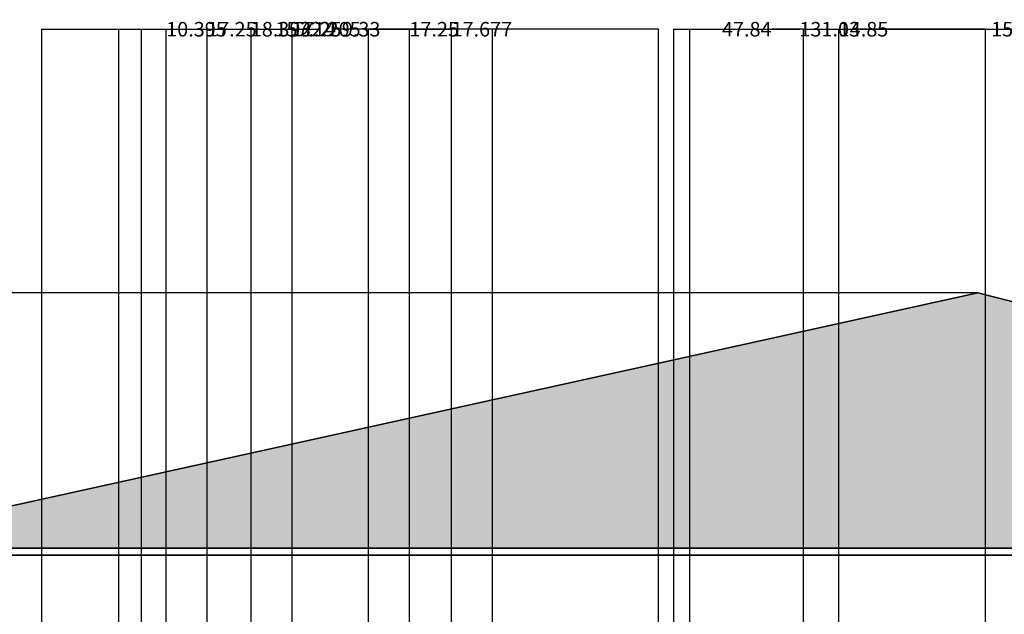
# Model space of a CAD drawing. Units: inches. Extents: x -655 to 499, y 20 to 616.
# Tile 5 of 7: x -409 to 5, y 365 to 616. Entities that reach past the tile are written whole.
import ezdxf

# ---------------------------------------------------------------- set-up
doc = ezdxf.new("R2010")
doc.units = ezdxf.units.IN
doc.header["$MEASUREMENT"] = 0
doc.layers.add('A-ANNO-DIMS', color=2, linetype='Continuous', lineweight=18)
doc.layers.add('A-ROOF', color=1, linetype='Continuous', lineweight=35)
doc.styles.get("Standard").update_dxf_attribs({"font": 'arial.ttf'})
doc.dimstyles.get("Standard").update_dxf_attribs({"dimtxt": 6.125, "dimasz": 0.18, "dimexe": 0.18, "dimexo": 0.0625, "dimgap": 0.09, "dimtad": 0, "dimtih": 1, "dimtoh": 1, "dimdec": 4, "dimzin": 0, "dimdsep": 46, "dimlunit": 4, "dimtxsty": 'Standard', "dimcen": 0.09, "dimadec": 0, "dimazin": 0, "dimtfac": 1, "dimtdec": 4, "dimtofl": 0, "dimtmove": 0, "dimatfit": 3, "dimfxl": 1, "dimtolj": 1, "dimtzin": 0, "dimarcsym": 0})

# ---------------------------------------------------------------- blocks, each defined once
blk = doc.blocks.new('*D10')
at = {"layer": 'A-ANNO-DIMS', "color": 0, "lineweight": -2, "transparency": 16777216}
for p, q in [((434.11, 393.11), (434.11, 23.7)), ((-590.16, 75.57), (-590.16, 23.7)), ((-589.98, 23.88), (-90.54, 23.88)), ((433.93, 23.88), (-65.51, 23.88))]:
    blk.add_line(p, q, dxfattribs=at)
at = {"layer": 'A-ANNO-DIMS', "color": 0, "transparency": 16777216}
for points in [[(-589.98, 23.91), (-589.98, 23.85), (-590.16, 23.88)], [(433.93, 23.91), (433.93, 23.85), (434.11, 23.88)]]:
    blk.add_solid(points, dxfattribs=at)
at = {"layer": 'Defpoints', "color": 0, "transparency": 16777216}
for p in [(434.11, 393.17), (-590.16, 75.63), (434.11, 23.88)]:
    blk.add_point(p, dxfattribs=at)
at = {"layer": 'A-ANNO-DIMS', "color": 0, "transparency": 16777216, "insert": (-78.02, 23.88), "char_height": 6.125, "attachment_point": 5}
blk.add_mtext('\\A1;1024.3', dxfattribs=at)
blk = doc.blocks.new('*D17')
at = {"layer": 'A-ANNO-DIMS', "color": 0, "lineweight": -2, "transparency": 16777216}
for p, q in [((-399.38, 249.9), (-399.38, 611.71)), ((-399.2, 611.53), (-282.57, 611.53)), ((-140.23, 611.53), (-256.86, 611.53)), ((-140.05, 249.9), (-140.05, 611.71))]:
    blk.add_line(p, q, dxfattribs=at)
at = {"layer": 'A-ANNO-DIMS', "color": 0, "transparency": 16777216}
for points in [[(-399.2, 611.56), (-399.2, 611.5), (-399.38, 611.53)], [(-140.23, 611.56), (-140.23, 611.5), (-140.05, 611.53)]]:
    blk.add_solid(points, dxfattribs=at)
at = {"layer": 'Defpoints', "color": 0, "transparency": 16777216}
for p in [(-140.05, 611.53), (-399.38, 249.84), (-140.05, 249.84)]:
    blk.add_point(p, dxfattribs=at)
at = {"layer": 'A-ANNO-DIMS', "color": 0, "transparency": 16777216, "insert": (-269.71, 611.53), "char_height": 6.125, "attachment_point": 5}
blk.add_mtext('\\A1;259.33', dxfattribs=at)
blk = doc.blocks.new('*D21')
at = {"layer": 'A-ANNO-DIMS', "color": 0, "lineweight": -2, "transparency": 16777216}
for p, q in [((179.11, 559.78), (486.04, 559.78)), ((485.86, 559.6), (485.86, 320.92)), ((485.86, 75.81), (485.86, 314.49)), ((-590.1, 75.63), (486.04, 75.63))]:
    blk.add_line(p, q, dxfattribs=at)
at = {"layer": 'A-ANNO-DIMS', "color": 0, "transparency": 16777216}
for points in [[(485.83, 559.6), (485.89, 559.6), (485.86, 559.78)], [(485.83, 75.81), (485.89, 75.81), (485.86, 75.63)]]:
    blk.add_solid(points, dxfattribs=at)
at = {"layer": 'Defpoints', "color": 0, "transparency": 16777216}
for p in [(179.05, 559.78), (485.86, 559.78), (-590.16, 75.63)]:
    blk.add_point(p, dxfattribs=at)
at = {"layer": 'A-ANNO-DIMS', "color": 0, "transparency": 16777216, "insert": (485.86, 317.7), "char_height": 6.125, "attachment_point": 5}
blk.add_mtext('\\A1;484.15', dxfattribs=at)
blk = doc.blocks.new('*D22')
at = {"layer": 'A-ANNO-DIMS', "color": 0, "lineweight": -2, "transparency": 16777216}
for p, q in [((-5.81, 500.52), (-642.09, 500.52)), ((-641.91, 500.34), (-641.91, 450.03)), ((-641.91, 393.29), (-641.91, 443.6)), ((-493.1, 393.11), (-642.09, 393.11))]:
    blk.add_line(p, q, dxfattribs=at)
at = {"layer": 'A-ANNO-DIMS', "color": 0, "transparency": 16777216}
for points in [[(-641.94, 500.34), (-641.88, 500.34), (-641.91, 500.52)], [(-641.94, 393.29), (-641.88, 393.29), (-641.91, 393.11)]]:
    blk.add_solid(points, dxfattribs=at)
at = {"layer": 'Defpoints', "color": 0, "transparency": 16777216}
for p in [(-641.91, 500.52), (-5.74, 500.52), (-493.03, 393.11)]:
    blk.add_point(p, dxfattribs=at)
at = {"layer": 'A-ANNO-DIMS', "color": 0, "transparency": 16777216, "insert": (-641.91, 446.81), "char_height": 6.125, "attachment_point": 5}
blk.add_mtext('\\A1;107.41', dxfattribs=at)
blk = doc.blocks.new('*D27')
at = {"layer": 'A-ANNO-DIMS', "color": 0, "lineweight": -2, "transparency": 16777216}
for p, q in [((-357.43, 359.35), (-357.43, 611.71)), ((-357.25, 611.53), (-347.21, 611.53)), ((-347.03, 350.2), (-347.03, 611.71)), ((-347.03, 611.53), (-346.85, 611.53))]:
    blk.add_line(p, q, dxfattribs=at)
at = {"layer": 'A-ANNO-DIMS', "color": 0, "transparency": 16777216}
for points in [[(-357.25, 611.56), (-357.25, 611.5), (-357.43, 611.53)], [(-347.21, 611.56), (-347.21, 611.5), (-347.03, 611.53)]]:
    blk.add_solid(points, dxfattribs=at)
at = {"layer": 'Defpoints', "color": 0, "transparency": 16777216}
for p in [(-347.03, 611.53), (-357.43, 359.29), (-347.03, 350.13)]:
    blk.add_point(p, dxfattribs=at)
at = {"layer": 'A-ANNO-DIMS', "color": 0, "transparency": 16777216, "insert": (-334.32, 611.53), "char_height": 6.125, "attachment_point": 5}
blk.add_mtext('\\A1;10.395', dxfattribs=at)
blk = doc.blocks.new('*D28')
at = {"layer": 'A-ANNO-DIMS', "color": 0, "lineweight": -2, "transparency": 16777216}
for p, q in [((-347.03, 350.2), (-347.03, 611.71)), ((-346.85, 611.53), (-329.96, 611.53)), ((-329.78, 350.2), (-329.78, 611.71)), ((-329.78, 611.53), (-329.6, 611.53))]:
    blk.add_line(p, q, dxfattribs=at)
at = {"layer": 'A-ANNO-DIMS', "color": 0, "transparency": 16777216}
for points in [[(-346.85, 611.56), (-346.85, 611.5), (-347.03, 611.53)], [(-329.96, 611.56), (-329.96, 611.5), (-329.78, 611.53)]]:
    blk.add_solid(points, dxfattribs=at)
at = {"layer": 'Defpoints', "color": 0, "transparency": 16777216}
for p in [(-329.78, 611.53), (-347.03, 350.13), (-329.78, 350.13)]:
    blk.add_point(p, dxfattribs=at)
at = {"layer": 'A-ANNO-DIMS', "color": 0, "transparency": 16777216, "insert": (-319.44, 611.53), "char_height": 6.125, "attachment_point": 5}
blk.add_mtext('\\A1;17.25', dxfattribs=at)
blk = doc.blocks.new('*D29')
at = {"layer": 'A-ANNO-DIMS', "color": 0, "lineweight": -2, "transparency": 16777216}
for p, q in [((-329.78, 350.2), (-329.78, 611.71)), ((-329.6, 611.53), (-311.57, 611.53)), ((-311.39, 350.2), (-311.39, 611.71)), ((-311.39, 611.53), (-311.21, 611.53))]:
    blk.add_line(p, q, dxfattribs=at)
at = {"layer": 'A-ANNO-DIMS', "color": 0, "transparency": 16777216}
for points in [[(-329.6, 611.56), (-329.6, 611.5), (-329.78, 611.53)], [(-311.57, 611.56), (-311.57, 611.5), (-311.39, 611.53)]]:
    blk.add_solid(points, dxfattribs=at)
at = {"layer": 'Defpoints', "color": 0, "transparency": 16777216}
for p in [(-311.39, 611.53), (-329.78, 350.13), (-311.39, 350.13)]:
    blk.add_point(p, dxfattribs=at)
at = {"layer": 'A-ANNO-DIMS', "color": 0, "transparency": 16777216, "insert": (-298.73, 611.53), "char_height": 6.125, "attachment_point": 5}
blk.add_mtext('\\A1;18.392', dxfattribs=at)
blk = doc.blocks.new('*D30')
at = {"layer": 'A-ANNO-DIMS', "color": 0, "lineweight": -2, "transparency": 16777216}
for p, q in [((-311.39, 350.2), (-311.39, 611.71)), ((-311.21, 611.53), (-294.32, 611.53)), ((-294.14, 350.2), (-294.14, 611.71)), ((-294.14, 611.53), (-293.96, 611.53))]:
    blk.add_line(p, q, dxfattribs=at)
at = {"layer": 'A-ANNO-DIMS', "color": 0, "transparency": 16777216}
for points in [[(-311.21, 611.56), (-311.21, 611.5), (-311.39, 611.53)], [(-294.32, 611.56), (-294.32, 611.5), (-294.14, 611.53)]]:
    blk.add_solid(points, dxfattribs=at)
at = {"layer": 'Defpoints', "color": 0, "transparency": 16777216}
for p in [(-294.14, 611.53), (-311.39, 350.13), (-294.14, 350.13)]:
    blk.add_point(p, dxfattribs=at)
at = {"layer": 'A-ANNO-DIMS', "color": 0, "transparency": 16777216, "insert": (-283.8, 611.53), "char_height": 6.125, "attachment_point": 5}
blk.add_mtext('\\A1;17.25', dxfattribs=at)
blk = doc.blocks.new('*D31')
at = {"layer": 'A-ANNO-DIMS', "color": 0, "lineweight": -2, "transparency": 16777216}
for p, q in [((-294.14, 350.2), (-294.14, 611.71)), ((-293.96, 611.53), (-290.86, 611.53)), ((-262.12, 611.53), (-265.21, 611.53)), ((-261.94, 350.2), (-261.94, 611.71))]:
    blk.add_line(p, q, dxfattribs=at)
at = {"layer": 'A-ANNO-DIMS', "color": 0, "transparency": 16777216}
for points in [[(-293.96, 611.56), (-293.96, 611.5), (-294.14, 611.53)], [(-262.12, 611.56), (-262.12, 611.5), (-261.94, 611.53)]]:
    blk.add_solid(points, dxfattribs=at)
at = {"layer": 'Defpoints', "color": 0, "transparency": 16777216}
for p in [(-261.94, 611.53), (-294.14, 350.13), (-261.94, 350.13)]:
    blk.add_point(p, dxfattribs=at)
at = {"layer": 'A-ANNO-DIMS', "color": 0, "transparency": 16777216, "insert": (-278.04, 611.53), "char_height": 6.125, "attachment_point": 5}
blk.add_mtext('\\A1;32.205', dxfattribs=at)
blk = doc.blocks.new('*D32')
at = {"layer": 'A-ANNO-DIMS', "color": 0, "lineweight": -2, "transparency": 16777216}
for p, q in [((-261.94, 350.2), (-261.94, 611.71)), ((-261.76, 611.53), (-244.87, 611.53)), ((-244.69, 350.2), (-244.69, 611.71)), ((-244.69, 611.53), (-244.51, 611.53))]:
    blk.add_line(p, q, dxfattribs=at)
at = {"layer": 'A-ANNO-DIMS', "color": 0, "transparency": 16777216}
for points in [[(-261.76, 611.56), (-261.76, 611.5), (-261.94, 611.53)], [(-244.87, 611.56), (-244.87, 611.5), (-244.69, 611.53)]]:
    blk.add_solid(points, dxfattribs=at)
at = {"layer": 'Defpoints', "color": 0, "transparency": 16777216}
for p in [(-244.69, 611.53), (-261.94, 350.13), (-244.69, 350.13)]:
    blk.add_point(p, dxfattribs=at)
at = {"layer": 'A-ANNO-DIMS', "color": 0, "transparency": 16777216, "insert": (-234.35, 611.53), "char_height": 6.125, "attachment_point": 5}
blk.add_mtext('\\A1;17.25', dxfattribs=at)
blk = doc.blocks.new('*D33')
at = {"layer": 'A-ANNO-DIMS', "color": 0, "lineweight": -2, "transparency": 16777216}
for p, q in [((-244.69, 350.2), (-244.69, 611.71)), ((-244.51, 611.53), (-227.19, 611.53)), ((-227.01, 359.35), (-227.01, 611.71)), ((-227.01, 611.53), (-226.83, 611.53))]:
    blk.add_line(p, q, dxfattribs=at)
at = {"layer": 'A-ANNO-DIMS', "color": 0, "transparency": 16777216}
for points in [[(-244.51, 611.56), (-244.51, 611.5), (-244.69, 611.53)], [(-227.19, 611.56), (-227.19, 611.5), (-227.01, 611.53)]]:
    blk.add_solid(points, dxfattribs=at)
at = {"layer": 'Defpoints', "color": 0, "transparency": 16777216}
for p in [(-227.01, 611.53), (-227.01, 359.29), (-244.69, 350.13)]:
    blk.add_point(p, dxfattribs=at)
at = {"layer": 'A-ANNO-DIMS', "color": 0, "transparency": 16777216, "insert": (-214.31, 611.53), "char_height": 6.125, "attachment_point": 5}
blk.add_mtext('\\A1;17.677', dxfattribs=at)
blk = doc.blocks.new('*D43')
at = {"layer": 'A-ANNO-DIMS', "color": 0, "lineweight": -2, "transparency": 16777216}
for p, q in [((-366.94, 248.81), (-366.94, 611.71)), ((-366.76, 611.53), (-300.88, 611.53)), ((-209.98, 611.53), (-275.87, 611.53)), ((-209.8, 99.69), (-209.8, 611.71))]:
    blk.add_line(p, q, dxfattribs=at)
at = {"layer": 'A-ANNO-DIMS', "color": 0, "transparency": 16777216}
for points in [[(-366.76, 611.56), (-366.76, 611.5), (-366.94, 611.53)], [(-209.98, 611.56), (-209.98, 611.5), (-209.8, 611.53)]]:
    blk.add_solid(points, dxfattribs=at)
at = {"layer": 'Defpoints', "color": 0, "transparency": 16777216}
for p in [(-209.8, 611.53), (-366.94, 248.74), (-209.8, 99.63)]:
    blk.add_point(p, dxfattribs=at)
at = {"layer": 'A-ANNO-DIMS', "color": 0, "transparency": 16777216, "insert": (-288.37, 611.53), "char_height": 6.125, "attachment_point": 5}
blk.add_mtext('\\A1;157.14', dxfattribs=at)
blk = doc.blocks.new('*D55')
at = {"layer": 'A-ANNO-DIMS', "color": 0, "lineweight": -2, "transparency": 16777216}
for p, q in [((-133.53, 249.26), (-133.53, 611.71)), ((-133.35, 611.53), (-80.53, 611.53)), ((-2.68, 611.53), (-55.5, 611.53)), ((-2.5, 283.02), (-2.5, 611.71))]:
    blk.add_line(p, q, dxfattribs=at)
at = {"layer": 'A-ANNO-DIMS', "color": 0, "transparency": 16777216}
for points in [[(-133.35, 611.56), (-133.35, 611.5), (-133.53, 611.53)], [(-2.68, 611.56), (-2.68, 611.5), (-2.5, 611.53)]]:
    blk.add_solid(points, dxfattribs=at)
at = {"layer": 'Defpoints', "color": 0, "transparency": 16777216}
for p in [(-2.5, 611.53), (-2.5, 282.96), (-133.53, 249.2)]:
    blk.add_point(p, dxfattribs=at)
at = {"layer": 'A-ANNO-DIMS', "color": 0, "transparency": 16777216, "insert": (-68.01, 611.53), "char_height": 6.125, "attachment_point": 5}
blk.add_mtext('\\A1;131.03', dxfattribs=at)
blk = doc.blocks.new('*D56')
at = {"layer": 'A-ANNO-DIMS', "color": 0, "lineweight": -2, "transparency": 16777216}
for p, q in [((-2.5, 283.02), (-2.5, 611.71)), ((-2.32, 611.53), (46.26, 611.53)), ((115.13, 611.53), (66.55, 611.53)), ((115.31, 249.31), (115.31, 611.71))]:
    blk.add_line(p, q, dxfattribs=at)
at = {"layer": 'A-ANNO-DIMS', "color": 0, "transparency": 16777216}
for points in [[(-2.32, 611.56), (-2.32, 611.5), (-2.5, 611.53)], [(115.13, 611.56), (115.13, 611.5), (115.31, 611.53)]]:
    blk.add_solid(points, dxfattribs=at)
at = {"layer": 'Defpoints', "color": 0, "transparency": 16777216}
for p in [(115.31, 611.53), (-2.5, 282.96), (115.31, 249.25)]:
    blk.add_point(p, dxfattribs=at)
at = {"layer": 'A-ANNO-DIMS', "color": 0, "transparency": 16777216, "insert": (56.41, 611.53), "char_height": 6.125, "attachment_point": 5}
blk.add_mtext('\\A1;117.8', dxfattribs=at)
blk = doc.blocks.new('*D59')
at = {"layer": 'A-ANNO-DIMS', "color": 0, "lineweight": -2, "transparency": 16777216}
for p, q in [((-126.81, 243.69), (-126.81, 611.71)), ((-126.63, 611.53), (-113.42, 611.53)), ((-79.15, 611.53), (-92.35, 611.53)), ((-78.97, 243.69), (-78.97, 611.71))]:
    blk.add_line(p, q, dxfattribs=at)
at = {"layer": 'A-ANNO-DIMS', "color": 0, "transparency": 16777216}
for points in [[(-126.63, 611.56), (-126.63, 611.5), (-126.81, 611.53)], [(-79.15, 611.56), (-79.15, 611.5), (-78.97, 611.53)]]:
    blk.add_solid(points, dxfattribs=at)
at = {"layer": 'Defpoints', "color": 0, "transparency": 16777216}
for p in [(-78.97, 611.53), (-126.81, 243.63), (-78.97, 243.63)]:
    blk.add_point(p, dxfattribs=at)
at = {"layer": 'A-ANNO-DIMS', "color": 0, "transparency": 16777216, "insert": (-102.89, 611.53), "char_height": 6.125, "attachment_point": 5}
blk.add_mtext('\\A1;47.84', dxfattribs=at)
blk = doc.blocks.new('*D60')
at = {"layer": 'A-ANNO-DIMS', "color": 0, "lineweight": -2, "transparency": 16777216}
for p, q in [((-78.97, 243.69), (-78.97, 611.71)), ((-78.79, 611.53), (-64.3, 611.53)), ((-64.12, 233.34), (-64.12, 611.71)), ((-64.12, 611.53), (-63.94, 611.53))]:
    blk.add_line(p, q, dxfattribs=at)
at = {"layer": 'A-ANNO-DIMS', "color": 0, "transparency": 16777216}
for points in [[(-78.79, 611.56), (-78.79, 611.5), (-78.97, 611.53)], [(-64.3, 611.56), (-64.3, 611.5), (-64.12, 611.53)]]:
    blk.add_solid(points, dxfattribs=at)
at = {"layer": 'Defpoints', "color": 0, "transparency": 16777216}
for p in [(-64.12, 611.53), (-78.97, 243.63), (-64.12, 233.27)]:
    blk.add_point(p, dxfattribs=at)
at = {"layer": 'A-ANNO-DIMS', "color": 0, "transparency": 16777216, "insert": (-53.78, 611.53), "char_height": 6.125, "attachment_point": 5}
blk.add_mtext('\\A1;14.85', dxfattribs=at)
blk = doc.blocks.new('*D61')
at = {"layer": 'A-ANNO-DIMS', "color": 0, "lineweight": -2, "transparency": 16777216}
for p, q in [((-64.12, 233.34), (-64.12, 611.71)), ((-63.94, 611.53), (0.16, 611.53)), ((89.22, 611.53), (25.13, 611.53)), ((89.4, 243.69), (89.4, 611.71))]:
    blk.add_line(p, q, dxfattribs=at)
at = {"layer": 'A-ANNO-DIMS', "color": 0, "transparency": 16777216}
for points in [[(-63.94, 611.56), (-63.94, 611.5), (-64.12, 611.53)], [(89.22, 611.56), (89.22, 611.5), (89.4, 611.53)]]:
    blk.add_solid(points, dxfattribs=at)
at = {"layer": 'Defpoints', "color": 0, "transparency": 16777216}
for p in [(89.4, 611.53), (89.4, 243.63), (-64.12, 233.27)]:
    blk.add_point(p, dxfattribs=at)
at = {"layer": 'A-ANNO-DIMS', "color": 0, "transparency": 16777216, "insert": (12.64, 611.53), "char_height": 6.125, "attachment_point": 5}
blk.add_mtext('\\A1;153.52', dxfattribs=at)

msp = doc.modelspace()

# ---------------------------------------------------------------- hatches: boundary and pattern name
at = {"layer": 'A-ROOF'}
h = msp.add_hatch(dxfattribs=at)
h.set_pattern_fill('AR-RSHKE', color=256)
h.paths.add_polyline_path([(-5.7434, 500.5192), (-493.0344, 393.1054), (-371.042, 393.1054), (119.6374, 393.1054), (415.7378, 393.1651)])
h.paths.add_polyline_path([(119.638, 282.9577), (-2.4978, 282.9577), (-133.531, 249.2017), (115.3098, 249.2518), (119.638, 250.1911)])
h.paths.add_polyline_path([(270.6361, 282.9577), (119.638, 282.9577), (119.638, 250.1911)], flags=17)
h.paths.add_polyline_path([(270.6361, 282.9577), (119.638, 250.1911), (119.638, 249.2527), (395.6741, 249.3083)])
h.paths.add_polyline_path([(-493.0344, 269.4313), (-534.9108, 229.7008), (-493.0344, 229.7008)])

# ---------------------------------------------------------------- linework, layer by layer
for p, q in [((-493.0344, 393.1054), (-5.7434, 500.5192)), ((-5.7434, 500.5192), (415.7378, 393.1651)), ((-322.5736, 390.1054), (-491.0344, 390.1054)), ((119.6375, 390.1054), (-322.5736, 390.1054))]:
    msp.add_line(p, q, dxfattribs=at)
msp.add_lwpolyline([(432.6073, 393.1685), (119.6374, 393.1054), (-371.042, 393.1054), (-493.0344, 393.1054)], dxfattribs=at)

# ---------------------------------------------------------------- dimensions: what is measured, and where the dimension line sits
at = {"layer": 'A-ANNO-DIMS'}
for base, p1, p2, override, picture, middle in [((-140.0489, 611.5295), (-399.3758, 249.8418), (-140.0489, 249.8418), {"dimdec": 2, "dimlfac": 1, "dimrnd": 0, "dimzin": 0, "dimdsep": 46, "dimlunit": 2}, '*D17', (-269.7123, 611.5295)), ((-209.8047, 611.5295), (-366.9446, 248.7444), (-209.8047, 99.6296), {"dimdec": 2, "dimlfac": 1, "dimrnd": 0, "dimzin": 0, "dimdsep": 46, "dimlunit": 2}, '*D43', (-288.3746, 611.5295)), ((-347.0336, 611.5295), (-357.429, 359.2861), (-347.0336, 350.1333), {"dimdec": 3, "dimlfac": 1, "dimrnd": 0, "dimzin": 0, "dimdsep": 46, "dimlunit": 2}, '*D27', (-334.3152, 611.5295)), ((-329.7837, 611.5295), (-347.0336, 350.1333), (-329.7837, 350.1333), {"dimdec": 2, "dimlfac": 1, "dimrnd": 0, "dimzin": 0, "dimdsep": 46, "dimlunit": 2}, '*D28', (-319.4446, 611.5295)), ((-311.39124, 611.52951), (-329.78371, 350.13329), (-311.39124, 350.13329), {"dimdec": 3, "dimlfac": 1, "dimrnd": 0, "dimzin": 0, "dimdsep": 46, "dimlunit": 2}, '*D29', (-298.7271, 611.52951)), ((-294.1413, 611.5295), (-311.3912, 350.1333), (-294.1413, 350.1333), {"dimdec": 2, "dimlfac": 1, "dimrnd": 0, "dimzin": 0, "dimdsep": 46, "dimlunit": 2}, '*D30', (-283.8023, 611.5295)), ((-261.935835, 611.529514), (-294.141326, 350.133285), (-261.935835, 350.133285), {"dimdec": 3, "dimlfac": 1, "dimrnd": 0, "dimzin": 0, "dimdsep": 46, "dimlunit": 2}, '*D31', (-278.038581, 611.529514)), ((-244.6859, 611.5295), (-261.9358, 350.1333), (-244.6859, 350.1333), {"dimdec": 2, "dimlfac": 1, "dimrnd": 0, "dimzin": 0, "dimdsep": 46, "dimlunit": 2}, '*D32', (-234.3469, 611.5295)), ((-227.0087, 611.5295), (-244.6859, 350.1333), (-227.0087, 359.2861), {"dimdec": 3, "dimlfac": 1, "dimrnd": 0, "dimzin": 0, "dimdsep": 46, "dimlunit": 2}, '*D33', (-214.3132, 611.5295)), ((-2.4978, 611.5295), (-133.531, 249.2017), (-2.4978, 282.9577), {"dimdec": 2, "dimlfac": 1, "dimrnd": 0, "dimzin": 0, "dimdsep": 46, "dimlunit": 2}, '*D55', (-68.0144, 611.5295)), ((-78.9669, 611.5295), (-126.8077, 243.6296), (-78.9669, 243.6296), {"dimdec": 2, "dimlfac": 1, "dimrnd": 0, "dimzin": 0, "dimdsep": 46, "dimlunit": 2}, '*D59', (-102.8873, 611.5295)), ((-64.1158, 611.5295), (-78.9669, 243.6296), (-64.1158, 233.274), {"dimdec": 2, "dimlfac": 1, "dimrnd": 0, "dimzin": 0, "dimdsep": 46, "dimlunit": 2}, '*D60', (-53.7767, 611.5295)), ((89.4008, 611.5295), (-64.1158, 233.274), (89.4008, 243.6296), {"dimdec": 2, "dimlfac": 1, "dimrnd": 0, "dimzin": 0, "dimdsep": 46, "dimlunit": 2}, '*D61', (12.6425, 611.5295)), ((115.3098, 611.5295), (-2.4978, 282.9577), (115.3098, 249.2518), {"dimdec": 1, "dimlfac": 1, "dimrnd": 0, "dimzin": 0, "dimdsep": 46, "dimlunit": 2}, '*D56', (56.406, 611.5295)), ((434.1137, 23.8796), (-590.1625, 75.6296), (434.1137, 393.1688), {"dimdec": 1, "dimlfac": 1, "dimrnd": 0, "dimzin": 0, "dimdsep": 46, "dimlunit": 2}, '*D10', (-78.0244, 23.8796))]:
    dim = msp.add_linear_dim(base=base, p1=p1, p2=p2, dimstyle='Standard', override=override, dxfattribs=at)
    dim.commit()
    dim.dimension.update_dxf_attribs({"geometry": picture, "text_midpoint": middle})
for base, p1, p2, picture, middle in [((485.8637, 559.7795), (-590.1625, 75.6296), (179.0482, 559.7795), '*D21', (485.8637, 317.7046)), ((-641.9125, 500.5192), (-493.0344, 393.1054), (-5.7434, 500.5192), '*D22', (-641.9125, 446.8123))]:
    dim = msp.add_linear_dim(base=base, p1=p1, p2=p2, angle=90, dimstyle='Standard', override={"dimdec": 2, "dimlfac": 1, "dimrnd": 0, "dimzin": 0, "dimdsep": 46, "dimlunit": 2}, dxfattribs=at)
    dim.commit()
    dim.dimension.update_dxf_attribs({"geometry": picture, "text_midpoint": middle})

doc.saveas('drawing.dxf')
